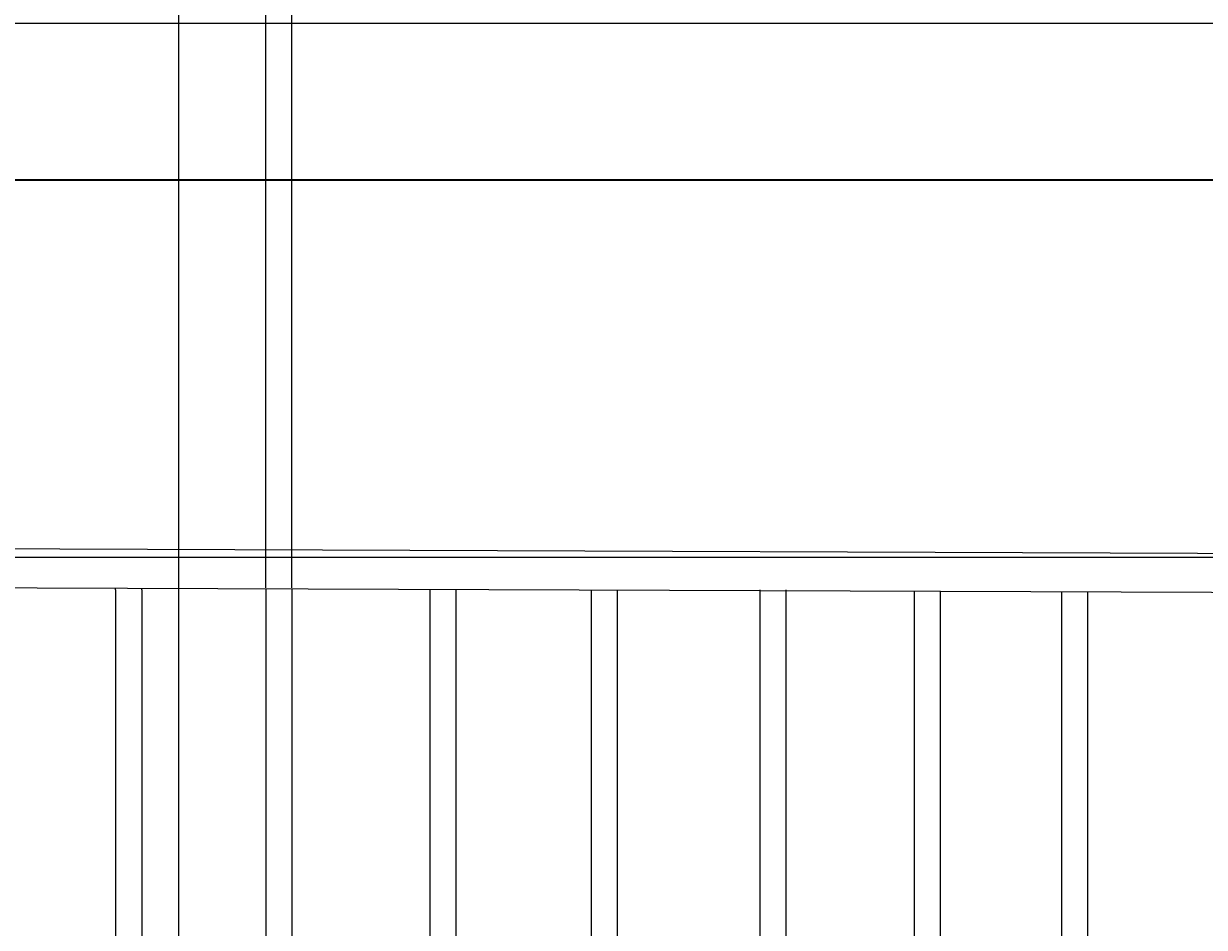
# Model space of a CAD drawing. Units: inches. Extents: x -13 to 809, y 112 to 656.
# Tile 21 of 55: x 430 to 521, y 181 to 251. Entities that reach past the tile are written whole.
import ezdxf

# ---------------------------------------------------------------- set-up
doc = ezdxf.new("R2010")
doc.units = ezdxf.units.IN
doc.header["$MEASUREMENT"] = 0
for name, color, linetype, lineweight in [('A-ANNO-DIMS', 2, 'Continuous', 18), ('A-DOOR', 4, 'Continuous', 25), ('A-ELEV', 7, 'Continuous', 35)]:
    doc.layers.add(name, color=color, linetype=linetype, lineweight=lineweight)
doc.styles.get("Standard").update_dxf_attribs({"font": 'arial.ttf'})
doc.dimstyles.get("Standard").update_dxf_attribs({"dimtxt": 0.625, "dimasz": 0.18, "dimexe": 0.18, "dimexo": 0.0625, "dimgap": 0.09, "dimtad": 0, "dimtih": 1, "dimtoh": 1, "dimdec": 4, "dimzin": 0, "dimdsep": 46, "dimlunit": 4, "dimtxsty": 'Standard', "dimcen": 0.09, "dimadec": 0, "dimazin": 0, "dimtfac": 1, "dimtdec": 4, "dimtofl": 0, "dimtmove": 0, "dimatfit": 3, "dimfxl": 1, "dimtolj": 1, "dimtzin": 0, "dimarcsym": 0})

# ---------------------------------------------------------------- blocks, each defined once
blk = doc.blocks.new('*D20')
at = {"layer": 'A-ANNO-DIMS', "color": 0, "lineweight": -2, "transparency": 16777216}
for p, q in [((365.938, 210.722), (365.938, 112.34)), ((607.574, 209.813), (607.574, 112.34)), ((366.118, 112.52), (485.365, 112.52)), ((607.394, 112.52), (488.148, 112.52))]:
    blk.add_line(p, q, dxfattribs=at)
at = {"layer": 'A-ANNO-DIMS', "color": 0, "transparency": 16777216}
for points in [[(366.118, 112.55), (366.118, 112.49), (365.938, 112.52)], [(607.394, 112.55), (607.394, 112.49), (607.574, 112.52)]]:
    blk.add_solid(points, dxfattribs=at)
at = {"layer": 'Defpoints', "color": 0, "transparency": 16777216}
for p in [(365.938, 210.785), (607.574, 209.875), (607.574, 112.52)]:
    blk.add_point(p, dxfattribs=at)
at = {"layer": 'A-ANNO-DIMS', "color": 0, "transparency": 16777216, "insert": (486.756, 112.52), "char_height": 0.625, "attachment_point": 5}
blk.add_mtext('\\A1;241.64', dxfattribs=at)
blk = doc.blocks.new('*D49')
at = {"layer": 'A-ANNO-DIMS', "color": 0, "lineweight": -2, "transparency": 16777216}
for p, q in [((590.946, 250.843), (-12.099, 250.843)), ((-11.919, 250.663), (-11.919, 245.247)), ((-11.919, 239.023), (-11.919, 244.439)), ((590.946, 238.843), (-12.099, 238.843))]:
    blk.add_line(p, q, dxfattribs=at)
at = {"layer": 'A-ANNO-DIMS', "color": 0, "transparency": 16777216}
for points in [[(-11.949, 250.663), (-11.889, 250.663), (-11.919, 250.843)], [(-11.949, 239.023), (-11.889, 239.023), (-11.919, 238.843)]]:
    blk.add_solid(points, dxfattribs=at)
at = {"layer": 'Defpoints', "color": 0, "transparency": 16777216}
for p in [(-11.919, 250.843), (591.008, 250.843), (591.008, 238.843)]:
    blk.add_point(p, dxfattribs=at)
at = {"layer": 'A-ANNO-DIMS', "color": 0, "transparency": 16777216, "insert": (-11.919, 244.843), "char_height": 0.625, "attachment_point": 5}
blk.add_mtext('\\A1;12', dxfattribs=at)
blk = doc.blocks.new('*D50')
at = {"layer": 'A-ANNO-DIMS', "color": 0, "lineweight": -2, "transparency": 16777216}
for p, q in [((590.946, 238.843), (-12.099, 238.843)), ((-11.919, 238.663), (-11.919, 224.768)), ((-11.919, 210.055), (-11.919, 223.95)), ((607.512, 209.875), (-12.099, 209.875))]:
    blk.add_line(p, q, dxfattribs=at)
at = {"layer": 'A-ANNO-DIMS', "color": 0, "transparency": 16777216}
for points in [[(-11.949, 238.663), (-11.889, 238.663), (-11.919, 238.843)], [(-11.949, 210.055), (-11.889, 210.055), (-11.919, 209.875)]]:
    blk.add_solid(points, dxfattribs=at)
at = {"layer": 'Defpoints', "color": 0, "transparency": 16777216}
for p in [(591.008, 238.843), (-11.919, 209.875), (607.574, 209.875)]:
    blk.add_point(p, dxfattribs=at)
at = {"layer": 'A-ANNO-DIMS', "color": 0, "transparency": 16777216, "insert": (-11.919, 224.359), "char_height": 0.625, "attachment_point": 5}
blk.add_mtext('\\A1;28.97', dxfattribs=at)
blk = doc.blocks.new('*D51')
at = {"layer": 'A-ANNO-DIMS', "color": 0, "lineweight": -2, "transparency": 16777216}
for p, q in [((341.407, 288.388), (341.407, 112.34)), ((442.184, 288.388), (442.184, 112.34)), ((341.587, 112.52), (390.437, 112.52)), ((442.004, 112.52), (393.154, 112.52))]:
    blk.add_line(p, q, dxfattribs=at)
at = {"layer": 'A-ANNO-DIMS', "color": 0, "transparency": 16777216}
for points in [[(341.587, 112.55), (341.587, 112.49), (341.407, 112.52)], [(442.004, 112.55), (442.004, 112.49), (442.184, 112.52)]]:
    blk.add_solid(points, dxfattribs=at)
at = {"layer": 'Defpoints', "color": 0, "transparency": 16777216}
for p in [(341.407, 288.451), (442.184, 288.451), (442.184, 112.52)]:
    blk.add_point(p, dxfattribs=at)
at = {"layer": 'A-ANNO-DIMS', "color": 0, "transparency": 16777216, "insert": (391.796, 112.52), "char_height": 0.625, "attachment_point": 5}
blk.add_mtext('\\A1;100.78', dxfattribs=at)
blk = doc.blocks.new('*D52')
at = {"layer": 'A-ANNO-DIMS', "color": 0, "lineweight": -2, "transparency": 16777216}
for p, q in [((442.184, 288.388), (442.184, 112.34)), ((542.962, 288.388), (542.962, 112.34)), ((442.364, 112.52), (491.215, 112.52)), ((542.782, 112.52), (493.932, 112.52))]:
    blk.add_line(p, q, dxfattribs=at)
at = {"layer": 'A-ANNO-DIMS', "color": 0, "transparency": 16777216}
for points in [[(442.364, 112.55), (442.364, 112.49), (442.184, 112.52)], [(542.782, 112.55), (542.782, 112.49), (542.962, 112.52)]]:
    blk.add_solid(points, dxfattribs=at)
at = {"layer": 'Defpoints', "color": 0, "transparency": 16777216}
for p in [(442.184, 288.451), (542.962, 288.451), (542.962, 112.52)]:
    blk.add_point(p, dxfattribs=at)
at = {"layer": 'A-ANNO-DIMS', "color": 0, "transparency": 16777216, "insert": (492.573, 112.52), "char_height": 0.625, "attachment_point": 5}
blk.add_mtext('\\A1;100.78', dxfattribs=at)
blk = doc.blocks.new('*D133')
at = {"layer": 'A-ANNO-DIMS', "color": 0, "lineweight": -2, "transparency": 16777216}
for p, q in [((448.701738, 655.782835), (448.521738, 655.782835)), ((448.881738, 207.535185), (448.881738, 655.962835)), ((450.881738, 207.527657), (450.881738, 655.962835)), ((451.061738, 655.782835), (451.241738, 655.782835))]:
    blk.add_line(p, q, dxfattribs=at)
at = {"layer": 'A-ANNO-DIMS', "color": 0, "transparency": 16777216}
for points in [[(448.701738, 655.812835), (448.701738, 655.752835), (448.881738, 655.782835)], [(451.061738, 655.812835), (451.061738, 655.752835), (450.881738, 655.782835)]]:
    blk.add_solid(points, dxfattribs=at)
at = {"layer": 'Defpoints', "color": 0, "transparency": 16777216}
for p in [(450.881738, 655.782835), (448.881738, 207.472685), (450.881738, 207.465157)]:
    blk.add_point(p, dxfattribs=at)
at = {"layer": 'A-ANNO-DIMS', "color": 0, "transparency": 16777216, "insert": (449.881738, 655.782835), "char_height": 0.625, "attachment_point": 5}
blk.add_mtext('\\A1;2.00', dxfattribs=at)

msp = doc.modelspace()

# ---------------------------------------------------------------- linework, layer by layer
at = {"layer": 'A-DOOR'}
for p, q in [((450.8817, 210.4727), (450.8817, 210.4652)), ((475.8241, 210.3788), (475.8241, 210.3713)), ((500.5957, 210.2856), (500.5957, 210.278)), ((511.8998, 210.243), (511.8998, 210.2355)), ((437.3579, 207.3724), (437.3584, 207.5161)), ((439.3579, 207.3724), (439.3584, 207.5085)), ((448.8817, 207.4727), (448.8817, 155.2141)), ((450.8817, 207.4652), (450.8817, 155.2141)), ((461.451, 207.3724), (461.4512, 207.4254)), ((463.451, 207.3724), (463.4511, 207.4178)), ((473.8241, 207.3788), (473.8241, 155.2141)), ((437.3579, 207.3724), (437.3579, 155.2141)), ((439.3579, 207.3724), (439.3579, 155.2141)), ((461.451, 207.3724), (461.451, 155.2141)), ((463.451, 207.3724), (463.451, 155.2141)), ((475.8241, 207.3713), (475.8241, 155.2141)), ((486.7562, 207.3724), (486.7562, 155.2141)), ((488.7562, 207.3724), (488.7562, 155.2141)), ((498.5957, 207.2855), (498.5957, 155.2141)), ((500.5957, 207.278), (500.5957, 155.2141)), ((509.8998, 207.243), (509.8998, 155.2141)), ((511.8998, 207.2355), (511.8998, 155.2141))]:
    msp.add_line(p, q, dxfattribs=at)
for points in [[(365.9383, 210.7849), (607.5741, 209.8753), (607.5741, 152.2141), (365.9383, 152.2141)], [(368.9383, 207.7736), (604.5741, 206.8866), (604.5741, 155.2141), (368.9383, 155.2141)]]:
    msp.add_lwpolyline(points, close=True, dxfattribs=at)
at = {"layer": 'A-ELEV'}
msp.add_line((341.4072, 238.8429), (591.008, 238.8429), dxfattribs=at)

# ---------------------------------------------------------------- dimensions: what is measured, and where the dimension line sits
at = {"layer": 'A-ANNO-DIMS'}
for base, p1, p2, picture, middle in [((450.8817, 655.7828), (448.8817, 207.4727), (450.8817, 207.4652), '*D133', (449.8817, 655.7828)), ((442.1845, 112.5199), (341.4072, 288.4508), (442.1845, 288.4508), '*D51', (391.7958, 112.5199)), ((542.9617, 112.5199), (442.1845, 288.4508), (542.9617, 288.4508), '*D52', (492.5731, 112.5199)), ((607.5741, 112.5199), (365.9383, 210.7849), (607.5741, 209.8753), '*D20', (486.7562, 112.5199))]:
    dim = msp.add_linear_dim(base=base, p1=p1, p2=p2, dimstyle='Standard', override={"dimdec": 2, "dimlfac": 1, "dimrnd": 0, "dimzin": 0, "dimdsep": 46, "dimlunit": 2}, dxfattribs=at)
    dim.commit()
    dim.dimension.update_dxf_attribs({"geometry": picture, "text_midpoint": middle})
for base, p2, override, picture, middle in [((-11.9191, 250.8429), (591.008, 250.8429), {"dimdec": 0, "dimlfac": 1, "dimrnd": 0, "dimzin": 0, "dimdsep": 46, "dimlunit": 2}, '*D49', (-11.9191, 244.8429)), ((-11.9191, 209.8753), (607.5741, 209.8753), {"dimdec": 2, "dimlfac": 1, "dimrnd": 0, "dimzin": 0, "dimdsep": 46, "dimlunit": 2}, '*D50', (-11.9191, 224.3591))]:
    dim = msp.add_linear_dim(base=base, p1=(591.008, 238.8429), p2=p2, angle=90, dimstyle='Standard', override=override, dxfattribs=at)
    dim.commit()
    dim.dimension.update_dxf_attribs({"geometry": picture, "text_midpoint": middle})

doc.saveas('drawing.dxf')
